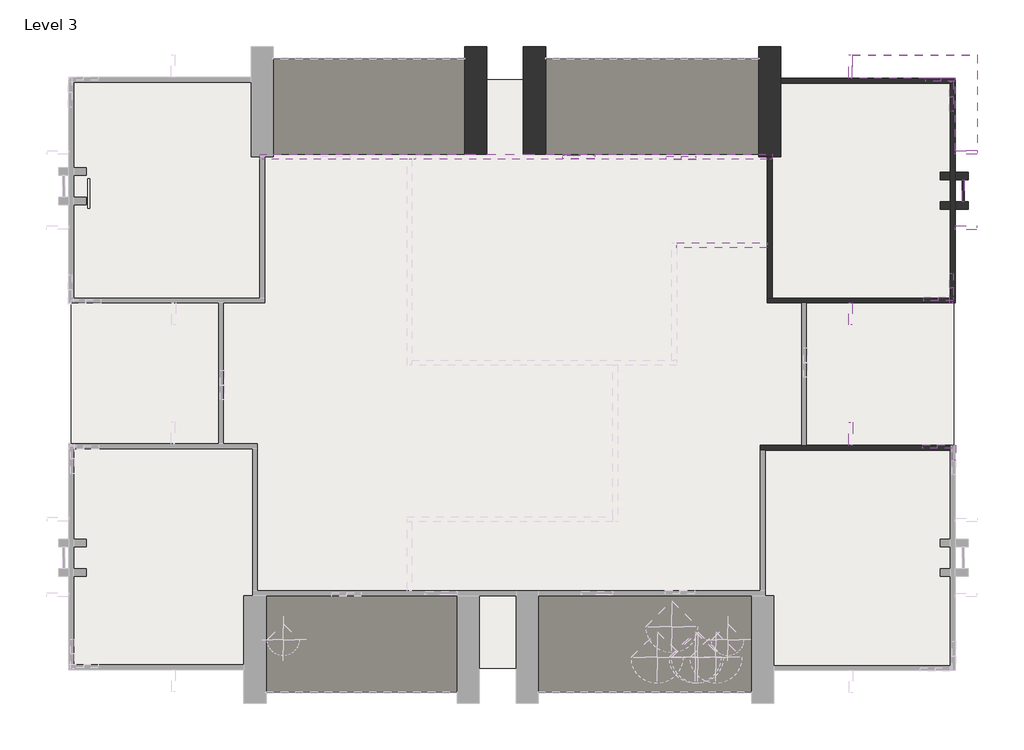
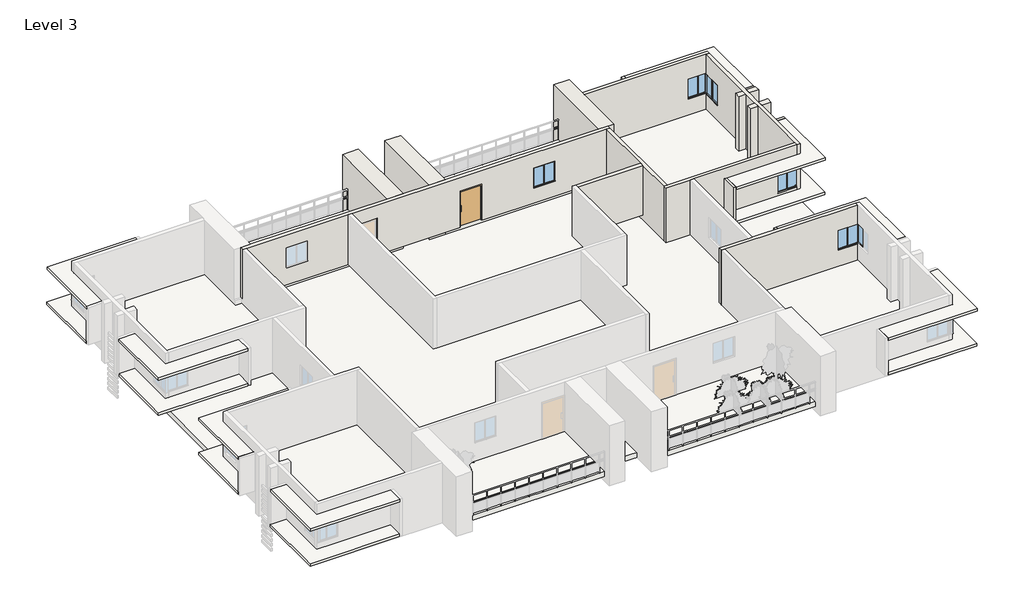
# One storey, part 3 of 4: 31 walls, 13 windows, 4 slabs, 1 door.
"""IFC4 building model written with IfcOpenShell, lengths in millimetres."""

from ifc_helpers import new_model, si_unit, frame, origin, place, context, project, spatial, polyline, outline, extrude, faceted_brep, transform, mapped, element, save
from components import door_15d3c954, window_20ff4747

model = new_model("IFC4")

# Units and contexts
model_context = context("Model", 3, world=origin())
ifc_project = project(units=[si_unit("LENGTHUNIT", "METRE", prefix="MILLI")], contexts=[model_context])

# Site, building, storey
site = spatial("IfcSite", under=ifc_project)
building = spatial("IfcBuilding", under=site)
storey = spatial("IfcBuildingStorey", under=building, Name="Level 3", Elevation=6096.0)

# Door
placement = place(None, origin())
door_shape = door_15d3c954(model_context)
element("IfcDoor", 1, ObjectType="Door-Passage-Single-Flush-Dbl_Acting : 48\" x 96\"", at=placement, inside=storey, context=model_context, shape_type="MappedRepresentation", body=[
    mapped(door_shape, transform((6249.0520665, 12804.5205944, 7315.2), x_axis=(1.0, 0.0, 0.0), y_axis=(0.0, 1.0, 0.0), z_axis=(0.0, 0.0, 1.0))),
])

# Slabs
element("IfcSlab", 2, ObjectType="Generic - 2'", at=placement, inside=storey, context=model_context, shape_type="SweptSolid", body=[
    extrude(outline(polyline([(21793.8520665, 16006.5548886), (21793.8520665, -8377.4451114), (-14782.1479335, -8377.4451114), (-14782.1479335, 16006.5548886), (21793.8520665, 16006.5548886)])), frame((0.0, 0.0, 6705.6), z_axis=(0.0, 0.0, 1.0), x_axis=(1.0, 0.0, 0.0)), (0.0, 0.0, 1.0), 304.8),
])
element("IfcSlab", 3, ObjectType="Generic - 2' gray", at=placement, inside=storey, context=model_context, shape_type="SweptSolid", body=[
    extrude(outline(polyline([(13411.8520665, -5363.830811), (13411.8520665, -9380.382663), (4572.6520665, -9380.382663), (4572.6520665, -5363.830811), (13411.8520665, -5363.830811)])), frame((0.0, 0.0, 7010.4), z_axis=(0.0, 0.0, 1.0), x_axis=(1.0, 0.0, 0.0)), (0.0, 0.0, 1.0), 304.8),
    extrude(outline(polyline([(-6704.9479335, -5363.1461695), (1219.8520665, -5363.1461695), (1219.8520665, -9380.382663), (-6704.9479335, -9380.382663), (-6704.9479335, -5363.1461695)])), frame((0.0, 0.0, 7010.4), z_axis=(0.0, 0.0, 1.0), x_axis=(1.0, 0.0, 0.0)), (0.0, 0.0, 1.0), 304.8),
    extrude(outline(polyline([(13716.6520665, 12912.4705944), (4877.4520665, 12912.4705944), (4877.4520665, 16886.1559451), (13716.6520665, 16886.1559451), (13716.6520665, 12912.4705944)])), frame((0.0, 0.0, 7010.4), z_axis=(0.0, 0.0, 1.0), x_axis=(1.0, 0.0, 0.0)), (0.0, 0.0, 1.0), 304.8),
    extrude(outline(polyline([(-6400.1479335, 12912.4705944), (-6400.1479335, 16886.1559451), (1524.6520665, 16886.1559451), (1524.6520665, 12912.4705944), (-6400.1479335, 12912.4705944)])), frame((0.0, 0.0, 7010.4), z_axis=(0.0, 0.0, 1.0), x_axis=(1.0, 0.0, 0.0)), (0.0, 0.0, 1.0), 304.8),
])
element("IfcSlab", 4, ObjectType="Generic - 6\"", at=placement, inside=storey, context=model_context, shape_type="SweptSolid", body=[
    extrude(outline(polyline([(-10616.5479335, -9354.6604699), (-15798.1479335, -9354.6604699), (-15798.1479335, -5392.2604699), (-14883.7479335, -5392.2604699), (-14883.7479335, -8338.6604699), (-14883.7479335, -8440.2604699), (-10616.5479335, -8440.2604699), (-10616.5479335, -9354.6604699)])), frame((0.0, 0.0, 7467.6), z_axis=(0.0, 0.0, 1.0), x_axis=(1.0, 0.0, 0.0)), (0.0, 0.0, 1.0), 152.4),
    extrude(outline(polyline([(-10633.1034654, 1834.0395301), (-10633.1034654, 919.6395301), (-14883.7479335, 919.6395301), (-14883.7479335, -2128.3604699), (-15775.8097154, -2128.3604699), (-15775.8097154, 1834.0395301), (-10633.1034654, 1834.0395301)])), frame((0.0, 0.0, 7467.6), z_axis=(0.0, 0.0, 1.0), x_axis=(1.0, 0.0, 0.0)), (0.0, 0.0, 1.0), 152.4),
    extrude(outline(polyline([(-10616.5479335, 5846.5548886), (-15798.1479335, 5846.5548886), (-15798.1479335, 9808.9548886), (-14883.7479335, 9808.9548886), (-14883.7479335, 6862.5548886), (-14883.7479335, 6760.9548886), (-10616.5479335, 6760.9548886), (-10616.5479335, 5846.5548886)])), frame((0.0, 0.0, 7467.6), z_axis=(0.0, 0.0, 1.0), x_axis=(1.0, 0.0, 0.0)), (0.0, 0.0, 1.0), 152.4),
    extrude(outline(polyline([(-10633.1034654, 17035.2548886), (-10633.1034654, 16120.8548886), (-14883.7479335, 16120.8548886), (-14883.7479335, 13072.8548886), (-15775.8097154, 13072.8548886), (-15775.8097154, 17035.2548886), (-10633.1034654, 17035.2548886)])), frame((0.0, 0.0, 7467.6), z_axis=(0.0, 0.0, 1.0), x_axis=(1.0, 0.0, 0.0)), (0.0, 0.0, 1.0), 152.4),
    extrude(outline(polyline([(17590.1520665, 17035.2548886), (22771.7520665, 17035.2548886), (22771.7520665, 13072.8548886), (21857.3520665, 13072.8548886), (21857.3520665, 16019.2548886), (21857.3520665, 16070.0548886), (17590.1520665, 16070.0548886), (17590.1520665, 16120.8548886), (17590.1520665, 17035.2548886)])), frame((0.0, 0.0, 7467.6), z_axis=(0.0, 0.0, 1.0), x_axis=(1.0, 0.0, 0.0)), (0.0, 0.0, 1.0), 152.4),
    extrude(outline(polyline([(17606.7075984, 5846.5548886), (17606.7075984, 6760.9548886), (21857.3520665, 6760.9548886), (21857.3520665, 9808.9548886), (22749.4138484, 9808.9548886), (22749.4138484, 5846.5548886), (17606.7075984, 5846.5548886)])), frame((0.0, 0.0, 7467.6), z_axis=(0.0, 0.0, 1.0), x_axis=(1.0, 0.0, 0.0)), (0.0, 0.0, 1.0), 152.4),
    extrude(outline(polyline([(17590.1520665, 1807.9548886), (22771.7520665, 1807.9548886), (22771.7520665, -2154.4451114), (21857.3520665, -2154.4451114), (21857.3520665, 791.9548886), (21857.3520665, 893.5548886), (17590.1520665, 893.5548886), (17590.1520665, 1807.9548886)])), frame((0.0, 0.0, 7467.6), z_axis=(0.0, 0.0, 1.0), x_axis=(1.0, 0.0, 0.0)), (0.0, 0.0, 1.0), 152.4),
    extrude(outline(polyline([(17606.7075984, -9380.7451114), (17606.7075984, -8466.3451114), (21857.3520665, -8466.3451114), (21857.3520665, -5418.3451114), (22749.4138484, -5418.3451114), (22749.4138484, -9380.7451114), (17606.7075984, -9380.7451114)])), frame((0.0, 0.0, 7467.6), z_axis=(0.0, 0.0, 1.0), x_axis=(1.0, 0.0, 0.0)), (0.0, 0.0, 1.0), 152.4),
])
element("IfcSlab", 5, ObjectType="Generic - 6\"", at=placement, inside=storey, context=model_context, shape_type="SweptSolid", body=[
    extrude(outline(polyline([(-10617.0810044, -9363.7552779), (-15798.6810044, -9363.7552779), (-15798.6810044, -5401.3552779), (-14884.2810044, -5401.3552779), (-14884.2810044, -8347.7552779), (-14884.2810044, -8449.3552779), (-10617.0810044, -8449.3552779), (-10617.0810044, -9363.7552779)])), frame((0.0, 0.0, 9601.2), z_axis=(0.0, 0.0, 1.0), x_axis=(1.0, 0.0, 0.0)), (0.0, 0.0, 1.0), 152.4),
    extrude(outline(polyline([(-10633.6365363, 1824.9447221), (-10633.6365363, 910.5447221), (-14884.2810044, 910.5447221), (-14884.2810044, -2137.4552779), (-15776.3427863, -2137.4552779), (-15776.3427863, 1824.9447221), (-10633.6365363, 1824.9447221)])), frame((0.0, 0.0, 9601.2), z_axis=(0.0, 0.0, 1.0), x_axis=(1.0, 0.0, 0.0)), (0.0, 0.0, 1.0), 152.4),
    extrude(outline(polyline([(-10617.0810044, 5837.4600805), (-15798.6810044, 5837.4600805), (-15798.6810044, 9799.8600805), (-14884.2810044, 9799.8600805), (-14884.2810044, 6853.4600805), (-14884.2810044, 6751.8600805), (-10617.0810044, 6751.8600805), (-10617.0810044, 5837.4600805)])), frame((0.0, 0.0, 9601.2), z_axis=(0.0, 0.0, 1.0), x_axis=(1.0, 0.0, 0.0)), (0.0, 0.0, 1.0), 152.4),
    extrude(outline(polyline([(-10633.6365363, 17026.1600805), (-10633.6365363, 16111.7600805), (-14884.2810044, 16111.7600805), (-14884.2810044, 13063.7600805), (-15776.3427863, 13063.7600805), (-15776.3427863, 17026.1600805), (-10633.6365363, 17026.1600805)])), frame((0.0, 0.0, 9601.2), z_axis=(0.0, 0.0, 1.0), x_axis=(1.0, 0.0, 0.0)), (0.0, 0.0, 1.0), 152.4),
    extrude(outline(polyline([(17589.6189956, 17026.1600805), (22771.2189956, 17026.1600805), (22771.2189956, 13063.7600805), (21856.8189956, 13063.7600805), (21856.8189956, 16010.1600805), (21856.8189956, 16060.9600805), (17589.6189956, 16060.9600805), (17589.6189956, 16111.7600805), (17589.6189956, 17026.1600805)])), frame((0.0, 0.0, 9601.2), z_axis=(0.0, 0.0, 1.0), x_axis=(1.0, 0.0, 0.0)), (0.0, 0.0, 1.0), 152.4),
    extrude(outline(polyline([(17606.1745274, 5837.4600805), (17606.1745274, 6751.8600805), (21856.8189956, 6751.8600805), (21856.8189956, 9799.8600805), (22748.8807774, 9799.8600805), (22748.8807774, 5837.4600805), (17606.1745274, 5837.4600805)])), frame((0.0, 0.0, 9601.2), z_axis=(0.0, 0.0, 1.0), x_axis=(1.0, 0.0, 0.0)), (0.0, 0.0, 1.0), 152.4),
    extrude(outline(polyline([(17589.6189956, 1798.8600805), (22771.2189956, 1798.8600805), (22771.2189956, -2163.5399195), (21856.8189956, -2163.5399195), (21856.8189956, 782.8600805), (21856.8189956, 884.4600805), (17589.6189956, 884.4600805), (17589.6189956, 1798.8600805)])), frame((0.0, 0.0, 9601.2), z_axis=(0.0, 0.0, 1.0), x_axis=(1.0, 0.0, 0.0)), (0.0, 0.0, 1.0), 152.4),
    extrude(outline(polyline([(17606.1745274, -9389.8399195), (17606.1745274, -8475.4399195), (21856.8189956, -8475.4399195), (21856.8189956, -5427.4399195), (22748.8807774, -5427.4399195), (22748.8807774, -9389.8399195), (17606.1745274, -9389.8399195)])), frame((0.0, 0.0, 9601.2), z_axis=(0.0, 0.0, 1.0), x_axis=(1.0, 0.0, 0.0)), (0.0, 0.0, 1.0), 152.4),
])

# Walls
element("IfcWall", 6, ObjectType="Generic - 1'", at=placement, inside=storey, context=model_context, shape_type="SweptSolid", body=[
    extrude(outline(polyline([(22386.1027846, 11871.0705944), (21857.3520665, 11871.0705944), (21857.3520665, 12175.8705944), (22386.1027846, 12175.8705944), (22386.1027846, 11871.0705944)])), frame((0.0, 0.0, 6705.6), z_axis=(0.0, 0.0, 1.0), x_axis=(1.0, 0.0, 0.0)), (0.0, 0.0, 1.0), 3657.6),
])
element("IfcWall", 7, ObjectType="Generic - 1'", at=placement, inside=storey, context=model_context, shape_type="SweptSolid", body=[
    extrude(outline(polyline([(21235.7605971, 12175.8705944), (21654.1520665, 12175.8705944), (21654.1520665, 11871.0705944), (21235.7605971, 11871.0705944), (21235.7605971, 12175.8705944)])), frame((0.0, 0.0, 6705.6), z_axis=(0.0, 0.0, 1.0), x_axis=(1.0, 0.0, 0.0)), (0.0, 0.0, 1.0), 3657.6),
])
element("IfcWall", 8, ObjectType="Generic - 1'", at=placement, inside=storey, context=model_context, shape_type="SweptSolid", body=[
    extrude(outline(polyline([(22386.1027846, 10651.8705944), (21857.3520665, 10651.8705944), (21857.3520665, 10956.6705944), (22386.1027846, 10956.6705944), (22386.1027846, 10651.8705944)])), frame((0.0, 0.0, 6705.6), z_axis=(0.0, 0.0, 1.0), x_axis=(1.0, 0.0, 0.0)), (0.0, 0.0, 1.0), 3657.6),
])
element("IfcWall", 9, ObjectType="Generic - 1'", at=placement, inside=storey, context=model_context, shape_type="SweptSolid", body=[
    extrude(outline(polyline([(21235.7605971, 10956.6705944), (21654.1520665, 10956.6705944), (21654.1520665, 10651.8705944), (21235.7605971, 10651.8705944), (21235.7605971, 10956.6705944)])), frame((0.0, 0.0, 6705.6), z_axis=(0.0, 0.0, 1.0), x_axis=(1.0, 0.0, 0.0)), (0.0, 0.0, 1.0), 3657.6),
])
element("IfcWall", 10, ObjectType="Generic - 3'", at=placement, inside=storey, context=model_context, shape_type="SweptSolid", body=[
    extrude(outline(polyline([(2439.0520665, 17382.8705944), (2439.0520665, 12912.4705944), (1524.6520665, 12912.4705944), (1524.6520665, 17382.8705944), (2439.0520665, 17382.8705944)])), frame((0.0, 0.0, 6705.6), z_axis=(0.0, 0.0, 1.0), x_axis=(1.0, 0.0, 0.0)), (0.0, 0.0, 1.0), 3657.6),
])
element("IfcWall", 11, ObjectType="Generic - 3'", at=placement, inside=storey, context=model_context, shape_type="SweptSolid", body=[
    extrude(outline(polyline([(4877.4520665, 17382.8705944), (4877.4520665, 12912.4705944), (3963.0520665, 12912.4705944), (3963.0520665, 17382.8705944), (4877.4520665, 17382.8705944)])), frame((0.0, 0.0, 6705.6), z_axis=(0.0, 0.0, 1.0), x_axis=(1.0, 0.0, 0.0)), (0.0, 0.0, 1.0), 3657.6),
])
element("IfcWall", 12, ObjectType="Generic - 3'", at=placement, inside=storey, context=model_context, shape_type="Brep", body=[
    faceted_brep([(14631.0520665, 12810.8705944, 6705.6), (14631.0520665, 15866.8548886, 6705.6), (14631.0520665, 16070.0548886, 6705.6), (14631.0520665, 17382.8705944, 6705.6), (14631.0520665, 17382.8705944, 10363.2), (14631.0520665, 16070.0548886, 10363.2), (14631.0520665, 15866.8548886, 10363.2), (14631.0520665, 12912.4705944, 10363.2), (14631.0520665, 12912.4705944, 7315.2), (14631.0520665, 12810.8705944, 7315.2), (13716.6520665, 12810.8705944, 6705.6), (13716.6520665, 12810.8705944, 7315.2), (13716.6520665, 12912.4705944, 7315.2), (13716.6520665, 12912.4705944, 10363.2), (13716.6520665, 17382.8705944, 10363.2), (13716.6520665, 17382.8705944, 6705.6), (14275.4520665, 12810.8705944, 6705.6), (14072.2520665, 12810.8705944, 6705.6), (14275.4520665, 12912.4705944, 10363.2), (14275.4520665, 12810.8705944, 7315.2), (14072.2520665, 12810.8705944, 7315.2), (14275.4520665, 12912.4705944, 7315.2)], [[[0, 1, 2, 3, 4, 5, 6, 7, 8, 9]], [[10, 11, 12, 13, 14, 15]], [[3, 2, 1, 0, 16, 17, 10, 15]], [[4, 3, 15, 14]], [[7, 6, 5, 4, 14, 13, 18]], [[0, 9, 19, 20, 11, 10, 17, 16]], [[8, 21, 12, 11, 20, 19, 9]], [[8, 7, 18, 13, 12, 21]]]),
])
element("IfcWall", 13, ObjectType="Generic - 5\"", at=placement, inside=storey, context=model_context, shape_type="SweptSolid", body=[
    extrude(outline(polyline([(22145.9857703, 10956.6705944), (22145.9857703, 11871.0705944), (22222.1857703, 11871.0705944), (22222.1857703, 10956.6705944), (22145.9857703, 10956.6705944)])), frame((0.0, 0.0, 5054.6), z_axis=(0.0, 0.0, 1.0), x_axis=(1.0, 0.0, 0.0)), (0.0, 0.0, 1.0), 152.8735856),
])
element("IfcWall", 14, ObjectType="Generic - 5\"", at=placement, inside=storey, context=model_context, shape_type="SweptSolid", body=[
    extrude(outline(polyline([(22145.9857703, 10956.6705944), (22145.9857703, 11871.0705944), (22222.1857703, 11871.0705944), (22222.1857703, 10956.6705944), (22145.9857703, 10956.6705944)])), frame((0.0, 0.0, 5359.4), z_axis=(0.0, 0.0, 1.0), x_axis=(1.0, 0.0, 0.0)), (0.0, 0.0, 1.0), 152.8735856),
])
element("IfcWall", 15, ObjectType="Generic - 5\"", at=placement, inside=storey, context=model_context, shape_type="SweptSolid", body=[
    extrude(outline(polyline([(22145.9857703, 10956.6705944), (22145.9857703, 11871.0705944), (22222.1857703, 11871.0705944), (22222.1857703, 10956.6705944), (22145.9857703, 10956.6705944)])), frame((0.0, 0.0, 5638.8), z_axis=(0.0, 0.0, 1.0), x_axis=(1.0, 0.0, 0.0)), (0.0, 0.0, 1.0), 152.8735856),
])
element("IfcWall", 16, ObjectType="Generic - 5\"", at=placement, inside=storey, context=model_context, shape_type="SweptSolid", body=[
    extrude(outline(polyline([(22145.9857703, 10956.6705944), (22145.9857703, 11871.0705944), (22222.1857703, 11871.0705944), (22222.1857703, 10956.6705944), (22145.9857703, 10956.6705944)])), frame((0.0, 0.0, 5943.6), z_axis=(0.0, 0.0, 1.0), x_axis=(1.0, 0.0, 0.0)), (0.0, 0.0, 1.0), 152.8735856),
])
element("IfcWall", 17, ObjectType="Generic - 5\"", at=placement, inside=storey, context=model_context, shape_type="SweptSolid", body=[
    extrude(outline(polyline([(22145.9857703, 10956.6705944), (22145.9857703, 11871.0705944), (22222.1857703, 11871.0705944), (22222.1857703, 10956.6705944), (22145.9857703, 10956.6705944)])), frame((0.0, 0.0, 6248.4), z_axis=(0.0, 0.0, 1.0), x_axis=(1.0, 0.0, 0.0)), (0.0, 0.0, 1.0), 152.8735856),
])
element("IfcWall", 18, ObjectType="Generic - 5\"", at=placement, inside=storey, context=model_context, shape_type="SweptSolid", body=[
    extrude(outline(polyline([(22145.9857703, 10956.6705944), (22145.9857703, 11871.0705944), (22222.1857703, 11871.0705944), (22222.1857703, 10956.6705944), (22145.9857703, 10956.6705944)])), frame((0.0, 0.0, 6553.2), z_axis=(0.0, 0.0, 1.0), x_axis=(1.0, 0.0, 0.0)), (0.0, 0.0, 1.0), 152.8735856),
])
element("IfcWall", 19, ObjectType="Generic - 5\"", at=placement, inside=storey, context=model_context, shape_type="SweptSolid", body=[
    extrude(outline(polyline([(22145.9857703, 10956.6705944), (22145.9857703, 11871.0705944), (22222.1857703, 11871.0705944), (22222.1857703, 10956.6705944), (22145.9857703, 10956.6705944)])), frame((0.0, 0.0, 6959.6), z_axis=(0.0, 0.0, 1.0), x_axis=(1.0, 0.0, 0.0)), (0.0, 0.0, 1.0), 152.8735856),
])
element("IfcWall", 20, ObjectType="Generic - 5\"", at=placement, inside=storey, context=model_context, shape_type="SweptSolid", body=[
    extrude(outline(polyline([(22145.9857703, 10956.6705944), (22145.9857703, 11871.0705944), (22222.1857703, 11871.0705944), (22222.1857703, 10956.6705944), (22145.9857703, 10956.6705944)])), frame((0.0, 0.0, 7239.0), z_axis=(0.0, 0.0, 1.0), x_axis=(1.0, 0.0, 0.0)), (0.0, 0.0, 1.0), 152.8735856),
])
element("IfcWall", 21, ObjectType="Generic - 5\"", at=placement, inside=storey, context=model_context, shape_type="SweptSolid", body=[
    extrude(outline(polyline([(22145.9857703, 10956.6705944), (22145.9857703, 11871.0705944), (22222.1857703, 11871.0705944), (22222.1857703, 10956.6705944), (22145.9857703, 10956.6705944)])), frame((0.0, 0.0, 7518.4), z_axis=(0.0, 0.0, 1.0), x_axis=(1.0, 0.0, 0.0)), (0.0, 0.0, 1.0), 152.8735856),
])
element("IfcWall", 22, ObjectType="Generic - 5\"", at=placement, inside=storey, context=model_context, shape_type="SweptSolid", body=[
    extrude(outline(polyline([(22145.9857703, 10956.6705944), (22145.9857703, 11871.0705944), (22222.1857703, 11871.0705944), (22222.1857703, 10956.6705944), (22145.9857703, 10956.6705944)])), frame((0.0, 0.0, 7823.2), z_axis=(0.0, 0.0, 1.0), x_axis=(1.0, 0.0, 0.0)), (0.0, 0.0, 1.0), 152.8735856),
])
element("IfcWall", 23, ObjectType="Generic - 5\"", at=placement, inside=storey, context=model_context, shape_type="SweptSolid", body=[
    extrude(outline(polyline([(22145.9857703, 10956.6705944), (22145.9857703, 11871.0705944), (22222.1857703, 11871.0705944), (22222.1857703, 10956.6705944), (22145.9857703, 10956.6705944)])), frame((0.0, 0.0, 8128.0), z_axis=(0.0, 0.0, 1.0), x_axis=(1.0, 0.0, 0.0)), (0.0, 0.0, 1.0), 152.8735856),
])
element("IfcWall", 24, ObjectType="Generic - 5\"", at=placement, inside=storey, context=model_context, shape_type="SweptSolid", body=[
    extrude(outline(polyline([(22145.9857703, 10956.6705944), (22145.9857703, 11871.0705944), (22222.1857703, 11871.0705944), (22222.1857703, 10956.6705944), (22145.9857703, 10956.6705944)])), frame((0.0, 0.0, 8407.4), z_axis=(0.0, 0.0, 1.0), x_axis=(1.0, 0.0, 0.0)), (0.0, 0.0, 1.0), 152.8735856),
])
element("IfcWall", 25, ObjectType="Generic - 6\"", at=placement, inside=storey, context=model_context, shape_type="SweptSolid", body=[
    extrude(outline(polyline([(22771.7520665, 12914.1048886), (21857.3520665, 12914.1048886), (21857.3520665, 13066.5048886), (22771.7520665, 13066.5048886), (22771.7520665, 12914.1048886)])), frame((0.0, 0.0, 7467.6), z_axis=(0.0, 0.0, 1.0), x_axis=(1.0, 0.0, 0.0)), (0.0, 0.0, 1.0), 2286.0),
])
element("IfcWall", 26, ObjectType="Generic - 6\"", at=placement, inside=storey, context=model_context, shape_type="SweptSolid", body=[
    extrude(outline(polyline([(17590.1520665, 17035.2548886), (17590.1520665, 16070.0548886), (17437.7520665, 16070.0548886), (17437.7520665, 17035.2548886), (17590.1520665, 17035.2548886)])), frame((0.0, 0.0, 7467.6), z_axis=(0.0, 0.0, 1.0), x_axis=(1.0, 0.0, 0.0)), (0.0, 0.0, 1.0), 2286.0),
])
element("IfcWall", 27, ObjectType="Generic - 6\"", at=placement, inside=storey, context=model_context, shape_type="SweptSolid", body=[
    extrude(outline(polyline([(22748.8807774, 9799.8600805), (21857.3520665, 9799.8600805), (21857.3520665, 9952.2600805), (22748.8807774, 9952.2600805), (22748.8807774, 9799.8600805)])), frame((0.0, 0.0, 7467.6), z_axis=(0.0, 0.0, 1.0), x_axis=(1.0, 0.0, 0.0)), (0.0, 0.0, 1.0), 2286.0),
])
element("IfcWall", 28, ObjectType="Generic - 6\"", at=placement, inside=storey, context=model_context, shape_type="SweptSolid", body=[
    extrude(outline(polyline([(17441.6075984, 5850.1600805), (17441.6075984, 6760.9548886), (17594.0075984, 6760.9548886), (17594.0075984, 5850.1600805), (17441.6075984, 5850.1600805)])), frame((0.0, 0.0, 7467.6), z_axis=(0.0, 0.0, 1.0), x_axis=(1.0, 0.0, 0.0)), (0.0, 0.0, 1.0), 2286.0),
])
element("IfcWall", 29, ObjectType="Generic - 6\"", at=placement, inside=storey, context=model_context, shape_type="SweptSolid", body=[
    extrude(outline(polyline([(17595.9689956, 1807.9548886), (17595.9689956, 868.1548886), (17443.5689956, 868.1548886), (17443.5689956, 1807.9548886), (17595.9689956, 1807.9548886)])), frame((0.0, 0.0, 7467.6), z_axis=(0.0, 0.0, 1.0), x_axis=(1.0, 0.0, 0.0)), (0.0, 0.0, 1.0), 2286.0),
])
element("IfcWall", 30, ObjectType="Generic - 8\"", at=placement, inside=storey, context=model_context, shape_type="SweptSolid", body=[
    extrude(outline(polyline([(14072.2520665, 9051.6705944), (10313.0520665, 9051.6705944), (10313.0520665, 9254.8705944), (14072.2520665, 9254.8705944), (14072.2520665, 9051.6705944)])), frame((0.0, 0.0, 7315.2), z_axis=(0.0, 0.0, 1.0), x_axis=(1.0, 0.0, 0.0)), (0.0, 0.0, 1.0), 3048.0),
])
element("IfcWall", 31, ObjectType="Generic - 8\" gray", at=placement, inside=storey, context=model_context, shape_type="Brep", body=[
    faceted_brep([(21857.3520665, 16070.0548886, 6705.6), (14631.0520665, 16070.0548886, 6705.6), (14631.0520665, 16070.0548886, 10363.2), (21857.3520665, 16070.0548886, 10363.2), (20634.9770665, 16070.0548886, 7977.8804451), (21854.1770665, 16070.0548886, 7977.8804451), (21854.1770665, 16070.0548886, 9197.0804451), (20634.9770665, 16070.0548886, 9197.0804451), (14631.0520665, 15866.8548886, 6705.6), (21654.1520665, 15866.8548886, 6705.6), (21857.3520665, 15866.8548886, 6705.6), (21857.3520665, 15866.8548886, 7959.7280277), (21857.3520665, 15866.8548886, 9178.9280277), (21857.3520665, 15866.8548886, 10363.2), (21654.1520665, 15866.8548886, 10363.2), (14631.0520665, 15866.8548886, 10363.2), (20634.9770665, 15866.8548886, 9197.0804451), (21854.1770665, 15866.8548886, 9197.0804451), (21854.1770665, 15866.8548886, 7977.8804451), (20634.9770665, 15866.8548886, 7977.8804451)], [[[0, 1, 2, 3], [4, 5, 6, 7]], [[8, 9, 10, 11, 12, 13, 14, 15], [16, 17, 18, 19]], [[1, 0, 10, 9, 8]], [[3, 2, 15, 14, 13]], [[0, 3, 13, 12, 11, 10]], [[2, 1, 8, 15]], [[18, 17, 6, 5]], [[18, 5, 4, 19]], [[16, 7, 6, 17]], [[19, 4, 7, 16]]]),
])
element("IfcWall", 32, ObjectType="Generic - 8\" gray", at=placement, inside=storey, context=model_context, shape_type="Brep", body=[
    faceted_brep([(21857.3520665, 6760.9548886, 6705.6), (21857.3520665, 10651.8705944, 6705.6), (21857.3520665, 10956.6705944, 6705.6), (21857.3520665, 11871.0705944, 6705.6), (21857.3520665, 12175.8705944, 6705.6), (21857.3520665, 15866.8548886, 6705.6), (21857.3520665, 15866.8548886, 7959.7280277), (21857.3520665, 14696.4442594, 7959.7280277), (21857.3520665, 14696.4442594, 9178.9280277), (21857.3520665, 15866.8548886, 9178.9280277), (21857.3520665, 15866.8548886, 10363.2), (21857.3520665, 12175.8705944, 10363.2), (21857.3520665, 11871.0705944, 10363.2), (21857.3520665, 10956.6705944, 10363.2), (21857.3520665, 10651.8705944, 10363.2), (21857.3520665, 6760.9548886, 10363.2), (21857.3520665, 7997.1026284, 7812.6947232), (21857.3520665, 6777.9026284, 7812.6947232), (21857.3520665, 6777.9026284, 9031.8947232), (21857.3520665, 7997.1026284, 9031.8947232), (21654.1520665, 15866.8548886, 6705.6), (21654.1520665, 12175.8705944, 6705.6), (21654.1520665, 11871.0705944, 6705.6), (21654.1520665, 10956.6705944, 6705.6), (21654.1520665, 10651.8705944, 6705.6), (21654.1520665, 6964.1548886, 6705.6), (21654.1520665, 6760.9548886, 6705.6), (21654.1520665, 6760.9548886, 7763.5450479), (21654.1520665, 6760.9548886, 8982.7450479), (21654.1520665, 6760.9548886, 10363.2), (21654.1520665, 6964.1548886, 10363.2), (21654.1520665, 10651.8705944, 10363.2), (21654.1520665, 10956.6705944, 10363.2), (21654.1520665, 11871.0705944, 10363.2), (21654.1520665, 12175.8705944, 10363.2), (21654.1520665, 15866.8548886, 10363.2), (21654.1520665, 15866.8548886, 9178.9280277), (21654.1520665, 14696.4442594, 9178.9280277), (21654.1520665, 14696.4442594, 7959.7280277), (21654.1520665, 15866.8548886, 7959.7280277), (21654.1520665, 6777.9026284, 7812.6947232), (21654.1520665, 7997.1026284, 7812.6947232), (21654.1520665, 7997.1026284, 9031.8947232), (21654.1520665, 6777.9026284, 9031.8947232)], [[[0, 1, 2, 3, 4, 5, 6, 7, 8, 9, 10, 11, 12, 13, 14, 15], [16, 17, 18, 19]], [[20, 21, 22, 23, 24, 25, 26, 27, 28, 29, 30, 31, 32, 33, 34, 35, 36, 37, 38, 39], [40, 41, 42, 43]], [[5, 4, 3, 2, 1, 0, 26, 25, 24, 23, 22, 21, 20]], [[15, 14, 13, 12, 11, 10, 35, 34, 33, 32, 31, 30, 29]], [[0, 15, 29, 28, 27, 26]], [[5, 20, 39, 6]], [[35, 10, 9, 36]], [[38, 7, 6, 39]], [[8, 7, 38, 37]], [[8, 37, 36, 9]], [[16, 41, 40, 17]], [[18, 43, 42, 19]], [[19, 42, 41, 16]], [[43, 18, 17, 40]]]),
])
element("IfcWall", 33, ObjectType="Generic - 8\" gray", at=placement, inside=storey, context=model_context, shape_type="Brep", body=[
    faceted_brep([(14072.2520665, 6760.9548886, 6705.6), (15481.9520665, 6760.9548886, 6705.6), (15685.1520665, 6760.9548886, 6705.6), (21654.1520665, 6760.9548886, 6705.6), (21654.1520665, 6760.9548886, 7763.5450479), (20541.6213445, 6760.9548886, 7763.5450479), (20541.6213445, 6760.9548886, 8982.7450479), (21654.1520665, 6760.9548886, 8982.7450479), (21654.1520665, 6760.9548886, 10363.2), (15685.1520665, 6760.9548886, 10363.2), (15481.9520665, 6760.9548886, 10363.2), (14072.2520665, 6760.9548886, 10363.2), (21654.1520665, 6964.1548886, 6705.6), (14275.4520665, 6964.1548886, 6705.6), (14072.2520665, 6964.1548886, 6705.6), (14072.2520665, 6964.1548886, 10363.2), (14275.4520665, 6964.1548886, 10363.2), (21654.1520665, 6964.1548886, 10363.2), (21654.1520665, 6964.1548886, 8982.7450479), (20541.6213445, 6964.1548886, 8982.7450479), (20541.6213445, 6964.1548886, 7763.5450479), (21654.1520665, 6964.1548886, 7763.5450479)], [[[0, 1, 2, 3, 4, 5, 6, 7, 8, 9, 10, 11]], [[12, 13, 14, 15, 16, 17, 18, 19, 20, 21]], [[3, 2, 1, 0, 14, 13, 12]], [[11, 10, 9, 8, 17, 16, 15]], [[3, 12, 21, 4]], [[17, 8, 7, 18]], [[0, 11, 15, 14]], [[4, 21, 20, 5]], [[6, 5, 20, 19]], [[6, 19, 18, 7]]]),
])
element("IfcWall", 34, ObjectType="Generic - 8\" gray", at=placement, inside=storey, context=model_context, shape_type="Brep", body=[
    faceted_brep([(13767.4520665, 664.9548886, 6705.6), (13970.6520665, 664.9548886, 6705.6), (21654.1520665, 664.9548886, 6705.6), (21654.1520665, 664.9548886, 7977.8804451), (20505.783383, 664.9548886, 7977.8804451), (20505.783383, 664.9548886, 9197.0804451), (21654.1520665, 664.9548886, 9197.0804451), (21654.1520665, 664.9548886, 10363.2), (13970.6520665, 664.9548886, 10363.2), (13767.4520665, 664.9548886, 10363.2), (21654.1520665, 868.1548886, 6705.6), (15685.1520665, 868.1548886, 6705.6), (15481.9520665, 868.1548886, 6705.6), (13767.4520665, 868.1548886, 6705.6), (13767.4520665, 868.1548886, 10363.2), (15481.9520665, 868.1548886, 10363.2), (15685.1520665, 868.1548886, 10363.2), (21654.1520665, 868.1548886, 10363.2), (21654.1520665, 868.1548886, 9197.0804451), (20505.783383, 868.1548886, 9197.0804451), (20505.783383, 868.1548886, 7977.8804451), (21654.1520665, 868.1548886, 7977.8804451), (21654.1520665, 859.364485, 7977.8804451), (21654.1520665, 859.364485, 9197.0804451)], [[[0, 1, 2, 3, 4, 5, 6, 7, 8, 9]], [[10, 11, 12, 13, 14, 15, 16, 17, 18, 19, 20, 21]], [[2, 1, 0, 13, 12, 11, 10]], [[9, 8, 7, 17, 16, 15, 14]], [[2, 10, 21, 22, 3]], [[17, 7, 6, 23, 18]], [[0, 9, 14, 13]], [[3, 22, 21, 20, 4]], [[5, 4, 20, 19]], [[5, 19, 18, 23, 6]]]),
])
element("IfcWall", 35, ObjectType="Generic - 8\" gray", at=placement, inside=storey, context=model_context, shape_type="Brep", body=[
    faceted_brep([(-6958.9479335, 12912.4705944, 10363.2), (-6400.1479335, 12912.4705944, 10363.2), (1524.6520665, 12912.4705944, 10363.2), (2439.0520665, 12912.4705944, 10363.2), (3963.0520665, 12912.4705944, 10363.2), (4877.4520665, 12912.4705944, 10363.2), (13716.6520665, 12912.4705944, 10363.2), (14275.4520665, 12912.4705944, 10363.2), (14275.4520665, 12912.4705944, 7315.2), (13716.6520665, 12912.4705944, 7315.2), (6909.4520665, 12912.4705944, 7315.2), (6909.4520665, 12912.4705944, 9550.4), (5588.6520665, 12912.4705944, 9550.4), (5588.6520665, 12912.4705944, 7315.2), (813.4520665, 12912.4705944, 7315.2), (813.4520665, 12912.4705944, 9550.4), (-507.3479335, 12912.4705944, 9550.4), (-507.3479335, 12912.4705944, 7315.2), (-6400.1479335, 12912.4705944, 7315.2), (-6958.9479335, 12912.4705944, 7315.2), (11102.1500799, 12912.4705944, 8234.4873953), (11102.1500799, 12912.4705944, 9453.6873953), (9882.9500799, 12912.4705944, 9453.6873953), (9882.9500799, 12912.4705944, 8234.4873953), (-3213.321881, 12912.4705944, 8360.6298362), (-3213.321881, 12912.4705944, 9579.8298362), (-4432.521881, 12912.4705944, 9579.8298362), (-4432.521881, 12912.4705944, 8360.6298362), (14275.4520665, 12709.2705944, 10363.2), (14072.2520665, 12709.2705944, 10363.2), (-659.7479335, 12709.2705944, 10363.2), (-862.9479335, 12709.2705944, 10363.2), (-6755.7479335, 12709.2705944, 10363.2), (-6958.9479335, 12709.2705944, 10363.2), (-6958.9479335, 12709.2705944, 7315.2), (-6755.7479335, 12709.2705944, 7315.2), (-862.9479335, 12709.2705944, 7315.2), (-659.7479335, 12709.2705944, 7315.2), (-507.3479335, 12709.2705944, 7315.2), (-507.3479335, 12709.2705944, 9550.4), (813.4520665, 12709.2705944, 9550.4), (813.4520665, 12709.2705944, 7315.2), (5588.6520665, 12709.2705944, 7315.2), (5588.6520665, 12709.2705944, 9550.4), (6909.4520665, 12709.2705944, 9550.4), (6909.4520665, 12709.2705944, 7315.2), (14072.2520665, 12709.2705944, 7315.2), (14275.4520665, 12709.2705944, 7315.2), (11102.1500799, 12709.2705944, 9453.6873953), (11102.1500799, 12709.2705944, 8234.4873953), (9882.9500799, 12709.2705944, 8234.4873953), (9882.9500799, 12709.2705944, 9453.6873953), (-3213.321881, 12709.2705944, 9579.8298362), (-3213.321881, 12709.2705944, 8360.6298362), (-4432.521881, 12709.2705944, 8360.6298362), (-4432.521881, 12709.2705944, 9579.8298362), (14275.4520665, 12810.8705944, 7315.2), (-6958.9479335, 12810.8705944, 7315.2)], [[[0, 1, 2, 3, 4, 5, 6, 7, 8, 9, 10, 11, 12, 13, 14, 15, 16, 17, 18, 19], [20, 21, 22, 23], [24, 25, 26, 27]], [[28, 29, 30, 31, 32, 33, 34, 35, 36, 37, 38, 39, 40, 41, 42, 43, 44, 45, 46, 47], [48, 49, 50, 51], [52, 53, 54, 55]], [[8, 56, 47, 46, 45, 10, 9]], [[34, 57, 19, 18, 17, 38, 37, 36, 35]], [[13, 42, 41, 14]], [[7, 6, 5, 4, 3, 2, 1, 0, 33, 32, 31, 30, 29, 28]], [[8, 7, 28, 47, 56]], [[0, 19, 57, 34, 33]], [[49, 20, 23, 50]], [[21, 20, 49, 48]], [[21, 48, 51, 22]], [[22, 51, 50, 23]], [[53, 24, 27, 54]], [[25, 24, 53, 52]], [[25, 52, 55, 26]], [[26, 55, 54, 27]], [[44, 11, 10, 45]], [[11, 44, 43, 12]], [[12, 43, 42, 13]], [[40, 15, 14, 41]], [[15, 40, 39, 16]], [[16, 39, 38, 17]]]),
])
element("IfcWall", 36, ObjectType="Generic - 8\" gray", at=placement, inside=storey, context=model_context, shape_type="Brep", body=[
    faceted_brep([(14275.4520665, 6964.1548886, 6705.6), (14275.4520665, 12810.8705944, 6705.6), (14275.4520665, 12810.8705944, 7315.2), (14275.4520665, 12709.2705944, 7315.2), (14275.4520665, 12709.2705944, 10363.2), (14275.4520665, 6964.1548886, 10363.2), (14072.2520665, 6964.1548886, 6705.6), (14072.2520665, 6964.1548886, 10363.2), (14072.2520665, 9051.6705944, 10363.2), (14072.2520665, 9254.8705944, 10363.2), (14072.2520665, 12709.2705944, 10363.2), (14072.2520665, 12709.2705944, 7315.2), (14072.2520665, 12810.8705944, 7315.2), (14072.2520665, 12810.8705944, 6705.6)], [[[0, 1, 2, 3, 4, 5]], [[6, 7, 8, 9, 10, 11, 12, 13]], [[1, 0, 6, 13]], [[5, 4, 10, 9, 8, 7]], [[0, 5, 7, 6]], [[2, 1, 13, 12]], [[11, 3, 2, 12]], [[4, 3, 11, 10]]]),
])

# Windows
window_shape = window_20ff4747(model_context)
element("IfcWindow", 37, ObjectType="Instance - Fixed : 24\" x 48\"", at=placement, inside=storey, context=model_context, shape_type="MappedRepresentation", body=[
    mapped(window_shape, transform((21587.4770665, 15968.4548886, 7063.4804451), x_axis=(1.0, 0.0, 0.0), y_axis=(0.0, 1.0, 0.0), z_axis=(0.0, 0.0, 1.0))),
])
element("IfcWindow", 38, ObjectType="Instance - Fixed : 24\" x 48\"", at=placement, inside=storey, context=model_context, shape_type="MappedRepresentation", body=[
    mapped(window_shape, transform((20977.8770665, 15968.4548886, 7063.4804451), x_axis=(1.0, 0.0, 0.0), y_axis=(0.0, 1.0, 0.0), z_axis=(0.0, 0.0, 1.0))),
])
element("IfcWindow", 39, ObjectType="Instance - Fixed : 24\" x 48\"", at=placement, inside=storey, context=model_context, shape_type="MappedRepresentation", body=[
    mapped(window_shape, transform((21755.7520665, 15648.9442594, 7045.3280277), x_axis=(0.0, 1.0, 0.0), y_axis=(-1.0, 0.0, 0.0), z_axis=(0.0, 0.0, 1.0))),
])
element("IfcWindow", 40, ObjectType="Instance - Fixed : 24\" x 48\"", at=placement, inside=storey, context=model_context, shape_type="MappedRepresentation", body=[
    mapped(window_shape, transform((21755.7520665, 15039.3442594, 7045.3280277), x_axis=(0.0, 1.0, 0.0), y_axis=(-1.0, 0.0, 0.0), z_axis=(0.0, 0.0, 1.0))),
])
element("IfcWindow", 41, ObjectType="Instance - Fixed : 24\" x 48\"", at=placement, inside=storey, context=model_context, shape_type="MappedRepresentation", body=[
    mapped(window_shape, transform((21458.283383, 766.5548886, 7063.4804451), x_axis=(1.0, 0.0, 0.0), y_axis=(0.0, 1.0, 0.0), z_axis=(0.0, 0.0, 1.0))),
])
element("IfcWindow", 42, ObjectType="Instance - Fixed : 24\" x 48\"", at=placement, inside=storey, context=model_context, shape_type="MappedRepresentation", body=[
    mapped(window_shape, transform((20848.683383, 766.5548886, 7063.4804451), x_axis=(1.0, 0.0, 0.0), y_axis=(0.0, 1.0, 0.0), z_axis=(0.0, 0.0, 1.0))),
])
element("IfcWindow", 43, ObjectType="Instance - Fixed : 24\" x 48\"", at=placement, inside=storey, context=model_context, shape_type="MappedRepresentation", body=[
    mapped(window_shape, transform((21755.7520665, 516.464485, 7063.4804451), x_axis=(0.0, -1.0, 0.0), y_axis=(1.0, 0.0, 0.0), z_axis=(0.0, 0.0, 1.0))),
])
element("IfcWindow", 44, ObjectType="Instance - Fixed : 24\" x 48\"", at=placement, inside=storey, context=model_context, shape_type="MappedRepresentation", body=[
    mapped(window_shape, transform((21755.7520665, 7730.4026284, 6898.2947232), x_axis=(0.0, 1.0, 0.0), y_axis=(-1.0, 0.0, 0.0), z_axis=(0.0, 0.0, 1.0))),
])
element("IfcWindow", 45, ObjectType="Instance - Fixed : 24\" x 48\"", at=placement, inside=storey, context=model_context, shape_type="MappedRepresentation", body=[
    mapped(window_shape, transform((21755.7520665, 7120.8026284, 6898.2947232), x_axis=(0.0, 1.0, 0.0), y_axis=(-1.0, 0.0, 0.0), z_axis=(0.0, 0.0, 1.0))),
])
element("IfcWindow", 46, ObjectType="Instance - Fixed : 24\" x 48\"", at=placement, inside=storey, context=model_context, shape_type="MappedRepresentation", body=[
    mapped(window_shape, transform((21494.1213445, 6862.5548886, 6849.1450479), x_axis=(1.0, 0.0, 0.0), y_axis=(0.0, 1.0, 0.0), z_axis=(0.0, 0.0, 1.0))),
])
element("IfcWindow", 47, ObjectType="Instance - Fixed : 24\" x 48\"", at=placement, inside=storey, context=model_context, shape_type="MappedRepresentation", body=[
    mapped(window_shape, transform((20884.5213445, 6862.5548886, 6849.1450479), x_axis=(1.0, 0.0, 0.0), y_axis=(0.0, 1.0, 0.0), z_axis=(0.0, 0.0, 1.0))),
])
element("IfcWindow", 48, ObjectType="Instance - Fixed : 24\" x 48\"", at=placement, inside=storey, context=model_context, shape_type="MappedRepresentation", body=[
    mapped(window_shape, transform((10149.6500799, 12810.8705944, 7320.0873953), x_axis=(-1.0, 0.0, 0.0), y_axis=(0.0, -1.0, 0.0), z_axis=(0.0, 0.0, 1.0))),
])
element("IfcWindow", 49, ObjectType="Instance - Fixed : 24\" x 48\"", at=placement, inside=storey, context=model_context, shape_type="MappedRepresentation", body=[
    mapped(window_shape, transform((10759.2500799, 12810.8705944, 7320.0873953), x_axis=(-1.0, 0.0, 0.0), y_axis=(0.0, -1.0, 0.0), z_axis=(0.0, 0.0, 1.0))),
])

save(model, "model.ifc")

# Revit data of these elements
# Type "Door-Passage-Single-Flush-Dbl_Acting : 48\" x 96\""
#   Type Mark = "12"
#   Assembly Code = "B2030200"
#   Analytic Construction = "Wooden"
#   Thickness = 0' - 1 3/4"
#   Thermal Resistance (R) = 2.5876 (h·ft²·°F)/BTU
#   Swing Angle [instance default] = 45.00°
#   Strike Height = 3' - 4"
#   Rough Width [instance default] = 4' - 4"
#   Rough Height [instance default] = 7' - 4"
#   MF Opening Height [instance default] = 0' - 4"
#   MF Opening Width [instance default] = 0' - 4"
#   Inset Calculate [instance default] = 0' - 4"
#   Masonry Inset [instance default] = 0' - 1"
#   Height = 7' - 0"
#   Width = 4' - 0"
#   Heat Transfer Coefficient (U) = 0.3865 BTU/(h·ft²·°F)
#   Masonry Frame Depth = 0' - 5 3/4"
#   Masonry Frame [instance default] = yes
#   Function = 1
#   Dry Wall Frame [instance default] = no
#   Panel Material = Wood - Birch
#   Frame Material = Metal - Paint Finish - Grey
#   Door Handle Material = Aluminum
#   Visual Light Transmittance = 0
#   Solar Heat Gain Coefficient = 0
#   Wall Closure = (empty or 0)
# Type "Generic - 2'"
#   Assembly Code = "B1010"
#   Function = 0
#   Layers, outside or top first: 1' - 0" "Metal - Painted - Grey" (function 1)
# Type "Generic - 2' gray"
#   Assembly Code = "B1010"
#   Function = 0
#   Layers, outside or top first: 1' - 0" "Rigid insulation" (function 1)
# Type "Generic - 6\""
#   Assembly Code = "B1010"
#   Function = 0
#   Layers, outside or top first: 0' - 6" "Metal - Painted - Grey" (function 1)
# Type "Generic - 1'"
#   Assembly Code = "B2010"
#   Layers, outside or top first: 1' - 0" "Metal - Painted - Grey" (function 1)
# Type "Generic - 3'"
#   Assembly Code = "B2010"
#   Layers, outside or top first: 3' - 0" "Metal - Painted - Grey" (function 1)
# Type "Generic - 5\""
#   Assembly Code = "B2010"
#   Layers, outside or top first: 0' - 3" "Oak Flooring" (function 1)
# Type "Generic - 6\""
#   Assembly Code = "B2010"
#   Layers, outside or top first: 0' - 6" "Metal - Painted - Grey" (function 1)
# Type "Generic - 8\""
#   Assembly Code = "B2010"
#   Layers, outside or top first: 0' - 8" no material (function 1)
# Type "Generic - 8\" gray"
#   Assembly Code = "B2010"
#   Layers, outside or top first: 0' - 8" "Parking Stripe" (function 1)
# Type "Instance - Fixed : 24\" x 48\""
#   Type Mark = "11"
#   Construction Type Id = "GSP4R"
#   Assembly Code = "B2020100"
#   Analytic Construction = "1/8 in Pilkington single glazing"
#   Visual Light Transmittance = 0.9
#   Thermal Resistance (R) = 0.8466 (h·ft²·°F)/BTU
#   Solar Heat Gain Coefficient = 0.86
#   Heat Transfer Coefficient (U) = 1.1812 BTU/(h·ft²·°F)
#   Height [instance default] = 4' - 0"
#   Default Sill Height = 3' - 0"
#   Width [instance default] = 2' - 0"
#   Window Inset = 0' - 2"
#   Define Thermal Properties by = 1
#   Glass Pane Material = Glass
#   Sash Material = Iron, Ductile
#   Wall Closure = (empty or 0)
# Element 1 (IfcDoor, "Door-Passage-Single-Flush-Dbl_Acting : 48\" x 96\"")
#   Swing Angle = 45.00°
#   Rough Width = 4' - 4"
#   Rough Height = 7' - 4"
#   Masonry Inset = 0' - 1"
#   MF Opening Width = 0' - 4"
#   MF Opening Height = 0' - 4"
#   Inset Calculate = 0' - 4"
#   Masonry Frame = yes
#   Dry Wall Frame = no
#   Phase Created = New Construction
#   Materials on its faces: "Aluminum", "Metal - Paint Finish - Grey", "Wood - Birch"
# Element 2 (IfcSlab, "Generic - 2'")
#   Height Offset From Level = 3' - 0"
#   Phase Created = New Construction
#   Materials on its faces: "Metal - Painted - Grey"
# Element 3 (IfcSlab, "Generic - 2' gray")
#   Height Offset From Level = 4' - 0"
#   Phase Created = New Construction
#   Materials on its faces: "Rigid insulation"
# Element 4 (IfcSlab, "Generic - 6\"")
#   built-in parameter 1001955 = -1.5708 (stored number, unit not read)
#   Height Offset From Level = 5' - 0"
#   Phase Created = New Construction
#   Materials on its faces: "Metal - Painted - Grey"
# Element 5 (IfcSlab, "Generic - 6\"")
#   built-in parameter 1001955 = -1.5708 (stored number, unit not read)
#   Height Offset From Level = 12' - 0"
#   Phase Created = New Construction
#   Materials on its faces: "Metal - Painted - Grey"
# Elements 6, 7, 8, 9 (IfcWall, "Generic - 1'")
#   built-in parameter 1001111 = 2' - 0"
#   Top Offset = 0' - 0"
#   Base Offset = 2' - 0"
#   Unconnected Height = 12' - 0"
#   wall height = 12' - 0"
#   Phase Created = New Construction
#   Base Constraint = Level 3
#   Materials on its faces: "Metal - Painted - Grey"
# Elements 10, 11, 12 (IfcWall, "Generic - 3'")
#   built-in parameter 1001111 = 2' - 0"
#   Top Offset = 0' - 0"
#   Base Offset = 2' - 0"
#   Unconnected Height = 12' - 0"
#   wall height = 12' - 0"
#   Phase Created = New Construction
#   Base Constraint = Level 3
#   Materials on its faces: "Metal - Painted - Grey", "EIFS, Exterior Insulation"
# Element 13 (IfcWall, "Generic - 5\"")
#   built-in parameter 1001111 = -3' - 5"
#   Top Offset = -12' - 10.98135"
#   Base Offset = -3' - 5"
#   wall height = 0' - 6.01865"
#   Phase Created = New Construction
#   Base Constraint = Level 3
#   Top Constraint = Level 4
#   Materials on its faces: "Oak Flooring"
# Element 14 (IfcWall, "Generic - 5\"")
#   built-in parameter 1001111 = -2' - 5"
#   Top Offset = -11' - 10.98135"
#   Base Offset = -2' - 5"
#   wall height = 0' - 6.01865"
#   Phase Created = New Construction
#   Base Constraint = Level 3
#   Top Constraint = Level 4
#   Materials on its faces: "Oak Flooring"
# Element 15 (IfcWall, "Generic - 5\"")
#   built-in parameter 1001111 = -1' - 6"
#   Top Offset = -10' - 11.98135"
#   Base Offset = -1' - 6"
#   wall height = 0' - 6.01865"
#   Phase Created = New Construction
#   Base Constraint = Level 3
#   Top Constraint = Level 4
#   Materials on its faces: "Oak Flooring"
# Element 16 (IfcWall, "Generic - 5\"")
#   built-in parameter 1001111 = -0' - 6"
#   Top Offset = -9' - 11.98135"
#   Base Offset = -0' - 6"
#   wall height = 0' - 6.01865"
#   Phase Created = New Construction
#   Base Constraint = Level 3
#   Top Constraint = Level 4
#   Materials on its faces: "Oak Flooring"
# Element 17 (IfcWall, "Generic - 5\"")
#   built-in parameter 1001111 = 0' - 6"
#   Top Offset = -8' - 11.98135"
#   Base Offset = 0' - 6"
#   wall height = 0' - 6.01865"
#   Phase Created = New Construction
#   Base Constraint = Level 3
#   Top Constraint = Level 4
#   Materials on its faces: "Oak Flooring"
# Element 18 (IfcWall, "Generic - 5\"")
#   built-in parameter 1001111 = 1' - 6"
#   Top Offset = -7' - 11.98135"
#   Base Offset = 1' - 6"
#   wall height = 0' - 6.01865"
#   Phase Created = New Construction
#   Base Constraint = Level 3
#   Top Constraint = Level 4
#   Materials on its faces: "Oak Flooring"
# Element 19 (IfcWall, "Generic - 5\"")
#   built-in parameter 1001111 = 2' - 10"
#   Top Offset = -6' - 7.98135"
#   Base Offset = 2' - 10"
#   wall height = 0' - 6.01865"
#   Phase Created = New Construction
#   Base Constraint = Level 3
#   Top Constraint = Level 4
#   Materials on its faces: "Oak Flooring"
# Element 20 (IfcWall, "Generic - 5\"")
#   built-in parameter 1001111 = 3' - 9"
#   Top Offset = -5' - 8.98135"
#   Base Offset = 3' - 9"
#   wall height = 0' - 6.01865"
#   Phase Created = New Construction
#   Base Constraint = Level 3
#   Top Constraint = Level 4
#   Materials on its faces: "Oak Flooring"
# Element 21 (IfcWall, "Generic - 5\"")
#   built-in parameter 1001111 = 4' - 8"
#   Top Offset = -4' - 9.98135"
#   Base Offset = 4' - 8"
#   wall height = 0' - 6.01865"
#   Phase Created = New Construction
#   Base Constraint = Level 3
#   Top Constraint = Level 4
#   Materials on its faces: "Oak Flooring"
# Element 22 (IfcWall, "Generic - 5\"")
#   built-in parameter 1001111 = 5' - 8"
#   Top Offset = -3' - 9.98135"
#   Base Offset = 5' - 8"
#   wall height = 0' - 6.01865"
#   Phase Created = New Construction
#   Base Constraint = Level 3
#   Top Constraint = Level 4
#   Materials on its faces: "Oak Flooring"
# Element 23 (IfcWall, "Generic - 5\"")
#   built-in parameter 1001111 = 6' - 8"
#   Top Offset = -2' - 9.98135"
#   Base Offset = 6' - 8"
#   wall height = 0' - 6.01865"
#   Phase Created = New Construction
#   Base Constraint = Level 3
#   Top Constraint = Level 4
#   Materials on its faces: "Oak Flooring"
# Element 24 (IfcWall, "Generic - 5\"")
#   built-in parameter 1001111 = 7' - 7"
#   Top Offset = -1' - 10.98135"
#   Base Offset = 7' - 7"
#   wall height = 0' - 6.01865"
#   Phase Created = New Construction
#   Base Constraint = Level 3
#   Top Constraint = Level 4
#   Materials on its faces: "Oak Flooring"
# Elements 25, 26, 27, 28, 29 (IfcWall, "Generic - 6\"")
#   built-in parameter 1001111 = 4' - 6"
#   Top Offset = 0' - 0"
#   Base Offset = 4' - 6"
#   Unconnected Height = 7' - 6"
#   wall height = 7' - 6"
#   Phase Created = New Construction
#   Base Constraint = Level 3
#   Materials on its faces: "Metal - Painted - Grey"
# Element 30 (IfcWall, "Generic - 8\"")
#   built-in parameter 1001111 = 4' - 0"
#   Top Offset = 0' - 0"
#   Base Offset = 4' - 0"
#   Unconnected Height = 10' - 0"
#   wall height = 10' - 0"
#   Phase Created = New Construction
#   Base Constraint = Level 3
#   Materials on its faces: "Default Wall"
# Elements 31, 32, 33, 34, 36 (IfcWall, "Generic - 8\" gray")
#   built-in parameter 1001111 = 2' - 0"
#   Top Offset = 0' - 0"
#   Base Offset = 2' - 0"
#   Unconnected Height = 12' - 0"
#   wall height = 12' - 0"
#   Phase Created = New Construction
#   Base Constraint = Level 3
#   Materials on its faces: "Parking Stripe"
# Element 35 (IfcWall, "Generic - 8\" gray")
#   built-in parameter 1001111 = 4' - 0"
#   Top Offset = 0' - 0"
#   Base Offset = 4' - 0"
#   Unconnected Height = 10' - 0"
#   wall height = 10' - 0"
#   Phase Created = New Construction
#   Base Constraint = Level 3
#   Materials on its faces: "Parking Stripe"
# Element 37 (IfcWindow, "Instance - Fixed : 24\" x 48\"")
#   Mark = "47"
#   Width = 2' - 0"
#   Height = 4' - 0"
#   Phase Created = New Construction
#   Materials on its faces: "Iron, Ductile", "Glass"
# Element 38 (IfcWindow, "Instance - Fixed : 24\" x 48\"")
#   Mark = "48"
#   Width = 2' - 0"
#   Height = 4' - 0"
#   Phase Created = New Construction
#   Materials on its faces: "Iron, Ductile", "Glass"
# Element 39 (IfcWindow, "Instance - Fixed : 24\" x 48\"")
#   Mark = "49"
#   Width = 2' - 0"
#   Height = 4' - 0"
#   Phase Created = New Construction
#   Materials on its faces: "Iron, Ductile", "Glass"
# Element 40 (IfcWindow, "Instance - Fixed : 24\" x 48\"")
#   Mark = "50"
#   Width = 2' - 0"
#   Height = 4' - 0"
#   Phase Created = New Construction
#   Materials on its faces: "Iron, Ductile", "Glass"
# Element 41 (IfcWindow, "Instance - Fixed : 24\" x 48\"")
#   Mark = "51"
#   Width = 2' - 0"
#   Height = 4' - 0"
#   Phase Created = New Construction
#   Materials on its faces: "Iron, Ductile", "Glass"
# Element 42 (IfcWindow, "Instance - Fixed : 24\" x 48\"")
#   Mark = "52"
#   Width = 2' - 0"
#   Height = 4' - 0"
#   Phase Created = New Construction
#   Materials on its faces: "Iron, Ductile", "Glass"
# Element 43 (IfcWindow, "Instance - Fixed : 24\" x 48\"")
#   Mark = "54"
#   Width = 2' - 0"
#   Height = 4' - 0"
#   Phase Created = New Construction
#   Materials on its faces: "Iron, Ductile", "Glass"
# Element 44 (IfcWindow, "Instance - Fixed : 24\" x 48\"")
#   Mark = "75"
#   Width = 2' - 0"
#   Height = 4' - 0"
#   Phase Created = New Construction
#   Materials on its faces: "Iron, Ductile", "Glass"
# Element 45 (IfcWindow, "Instance - Fixed : 24\" x 48\"")
#   Mark = "76"
#   Width = 2' - 0"
#   Height = 4' - 0"
#   Phase Created = New Construction
#   Materials on its faces: "Iron, Ductile", "Glass"
# Element 46 (IfcWindow, "Instance - Fixed : 24\" x 48\"")
#   Mark = "77"
#   Width = 2' - 0"
#   Height = 4' - 0"
#   Phase Created = New Construction
#   Materials on its faces: "Iron, Ductile", "Glass"
# Element 47 (IfcWindow, "Instance - Fixed : 24\" x 48\"")
#   Mark = "78"
#   Width = 2' - 0"
#   Height = 4' - 0"
#   Phase Created = New Construction
#   Materials on its faces: "Iron, Ductile", "Glass"
# Element 48 (IfcWindow, "Instance - Fixed : 24\" x 48\"")
#   Mark = "79"
#   Width = 2' - 0"
#   Height = 4' - 0"
#   Phase Created = New Construction
#   Materials on its faces: "Iron, Ductile", "Glass"
# Element 49 (IfcWindow, "Instance - Fixed : 24\" x 48\"")
#   Mark = "80"
#   Width = 2' - 0"
#   Height = 4' - 0"
#   Phase Created = New Construction
#   Materials on its faces: "Iron, Ductile", "Glass"
# Materials
#   "Wood - Birch": class "Wood", colour RGB 166 116 52, transparency 0, Cost = 0
#   "Metal - Paint Finish - Grey": class "Paint", colour RGB 104 104 104, transparency 0, Cost = 0
#   "Aluminum": class "Metal", colour RGB 247 247 247, transparency 0, Description = "Aluminum 6061", Cost = 0
#   "Metal - Painted - Grey": class "Paint", colour RGB 104 104 104, transparency 0, Cost = 0
#   "Rigid insulation": class "Generic", colour RGB 127 127 127, transparency 0, Description = "Rigid foam insulation board", Cost = 0
#   "Oak Flooring": class "Wood", colour RGB 216 169 114, transparency 0, Description = "Quercus Rubra", Cost = 0
#   "Parking Stripe": class "Paint", colour RGB 250 250 91, transparency 0, Cost = 0
#   "Glass": class "Glass", colour RGB 0 128 192, transparency 0.75, Description = "Soda Lime Glass", Cost = 0
#   "Iron, Ductile": class "Metal", colour RGB 0 0 0, transparency 0, Description = "Ductile cast iron", Cost = 0
#   "EIFS, Exterior Insulation": class "Generic", colour RGB 127 127 127, transparency 0, Description = "EIFS - Exterior Insulation", Cost = 0
#   "Default Wall": colour RGB 128 128 128, transparency 0
